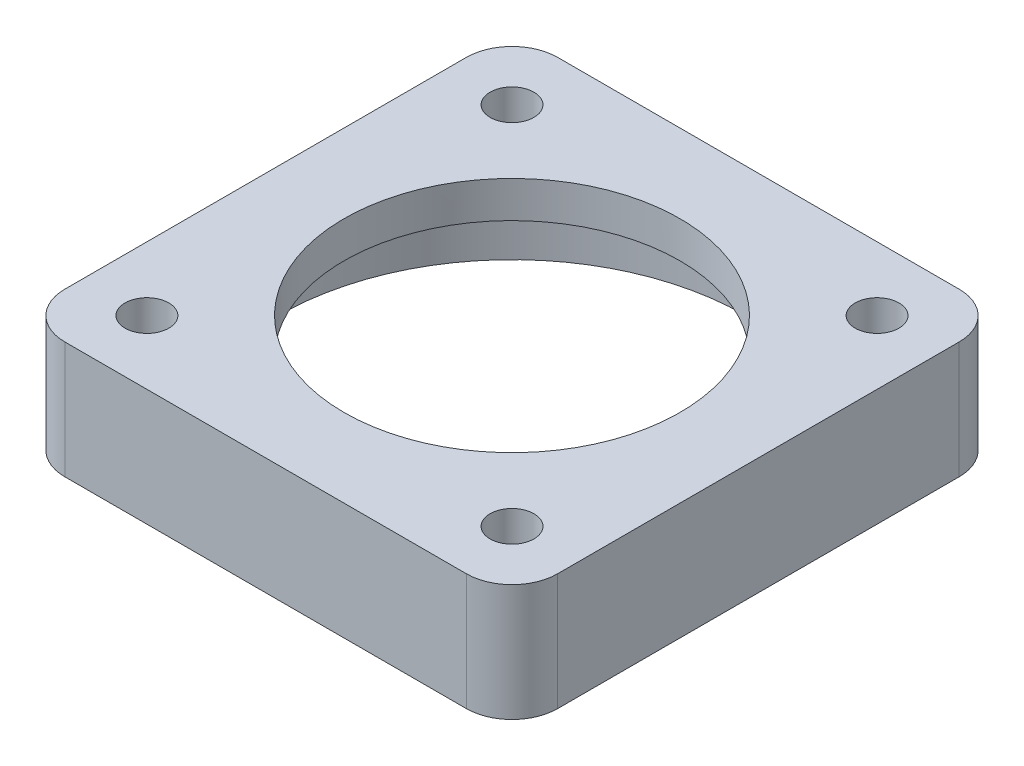
ISO-10303-21;
HEADER;
FILE_DESCRIPTION(('STEP AP214'),'2;1');
FILE_NAME('part.step','',(''),(''),'','','');
FILE_SCHEMA(('AUTOMOTIVE_DESIGN { 1 0 10303 214 1 1 1 1 }'));
ENDSEC;
DATA;
#1=APPLICATION_CONTEXT('core data for automotive mechanical design processes');
#2=APPLICATION_PROTOCOL_DEFINITION('international standard','automotive_design',2000,#1);
#3=PRODUCT_CONTEXT('',#1,'mechanical');
#4=PRODUCT('Part','Part','',(#3));
#5=PRODUCT_RELATED_PRODUCT_CATEGORY('part','',(#4));
#6=PRODUCT_DEFINITION_FORMATION('','',#4);
#7=PRODUCT_DEFINITION_CONTEXT('part definition',#1,'design');
#8=PRODUCT_DEFINITION('design','',#6,#7);
#9=PRODUCT_DEFINITION_SHAPE('','',#8);
#10=(LENGTH_UNIT() NAMED_UNIT(*) SI_UNIT(.MILLI.,.METRE.));
#11=(NAMED_UNIT(*) PLANE_ANGLE_UNIT() SI_UNIT($,.RADIAN.));
#12=(NAMED_UNIT(*) SI_UNIT($,.STERADIAN.) SOLID_ANGLE_UNIT());
#13=UNCERTAINTY_MEASURE_WITH_UNIT(LENGTH_MEASURE(1.E-05),#10,'distance_accuracy_value','');
#14=(GEOMETRIC_REPRESENTATION_CONTEXT(3) GLOBAL_UNCERTAINTY_ASSIGNED_CONTEXT((#13)) GLOBAL_UNIT_ASSIGNED_CONTEXT((#10,
#11,#12)) REPRESENTATION_CONTEXT('',''));
#15=CARTESIAN_POINT('',(0.,0.,0.));
#16=DIRECTION('',(0.,0.,1.));
#17=DIRECTION('',(1.,0.,0.));
#18=AXIS2_PLACEMENT_3D('',#15,#16,#17);
#19=CARTESIAN_POINT('',(0.,-0.001000000000001,0.));
#20=DIRECTION('',(0.,1.,0.));
#21=DIRECTION('',(0.,0.,1.));
#22=AXIS2_PLACEMENT_3D('',#19,#20,#21);
#23=CYLINDRICAL_SURFACE('',#22,46.);
#24=CARTESIAN_POINT('',(0.,32.,0.));
#25=DIRECTION('',(0.,1.,0.));
#26=DIRECTION('',(0.,0.,1.));
#27=AXIS2_PLACEMENT_3D('',#24,#25,#26);
#28=CIRCLE('',#27,46.);
#29=CARTESIAN_POINT('',(0.,32.,46.));
#30=VERTEX_POINT('',#29);
#31=EDGE_CURVE('E207',#30,#30,#28,.T.);
#32=ORIENTED_EDGE('',*,*,#31,.T.);
#33=EDGE_LOOP('',(#32));
#34=FACE_BOUND('',#33,.T.);
#35=CARTESIAN_POINT('',(0.,22.,0.));
#36=DIRECTION('',(0.,-1.,0.));
#37=DIRECTION('',(0.,0.,-1.));
#38=AXIS2_PLACEMENT_3D('',#35,#36,#37);
#39=CIRCLE('',#38,46.);
#40=CARTESIAN_POINT('',(0.,22.,-46.));
#41=VERTEX_POINT('',#40);
#42=EDGE_CURVE('E43',#41,#41,#39,.F.);
#43=ORIENTED_EDGE('',*,*,#42,.F.);
#44=EDGE_LOOP('',(#43));
#45=FACE_BOUND('',#44,.T.);
#46=ADVANCED_FACE('F39',(#34,#45),#23,.F.);
#47=CARTESIAN_POINT('',(-55.,32.,55.));
#48=DIRECTION('',(0.,1.,0.));
#49=DIRECTION('',(0.,0.,1.));
#50=AXIS2_PLACEMENT_3D('',#47,#48,#49);
#51=PLANE('',#50);
#52=ORIENTED_EDGE('',*,*,#31,.F.);
#53=EDGE_LOOP('',(#52));
#54=FACE_BOUND('',#53,.T.);
#55=CARTESIAN_POINT('',(50.0000000000001,32.,50.));
#56=DIRECTION('',(0.,1.,0.));
#57=DIRECTION('',(0.,0.,1.));
#58=AXIS2_PLACEMENT_3D('',#55,#56,#57);
#59=CIRCLE('',#58,5.99999999999999);
#60=CARTESIAN_POINT('',(50.0000000000001,32.,56.));
#61=VERTEX_POINT('',#60);
#62=EDGE_CURVE('E197',#61,#61,#59,.T.);
#63=ORIENTED_EDGE('',*,*,#62,.F.);
#64=EDGE_LOOP('',(#63));
#65=FACE_BOUND('',#64,.T.);
#66=CARTESIAN_POINT('',(-50.,32.,-50.));
#67=DIRECTION('',(0.,1.,0.));
#68=DIRECTION('',(0.,0.,1.));
#69=AXIS2_PLACEMENT_3D('',#66,#67,#68);
#70=CIRCLE('',#69,5.99999999999999);
#71=CARTESIAN_POINT('',(-50.,32.,-44.));
#72=VERTEX_POINT('',#71);
#73=EDGE_CURVE('E142',#72,#72,#70,.T.);
#74=ORIENTED_EDGE('',*,*,#73,.F.);
#75=EDGE_LOOP('',(#74));
#76=FACE_BOUND('',#75,.T.);
#77=CARTESIAN_POINT('',(-55.,32.,55.));
#78=DIRECTION('',(0.,1.,0.));
#79=DIRECTION('',(0.,0.,1.));
#80=AXIS2_PLACEMENT_3D('',#77,#78,#79);
#81=CIRCLE('',#80,12.5);
#82=CARTESIAN_POINT('',(-67.5,32.,55.));
#83=VERTEX_POINT('',#82);
#84=CARTESIAN_POINT('',(-55.,32.,67.5));
#85=VERTEX_POINT('',#84);
#86=EDGE_CURVE('E153',#83,#85,#81,.T.);
#87=ORIENTED_EDGE('',*,*,#86,.T.);
#88=DIRECTION('',(1.,0.,0.));
#89=VECTOR('',#88,1.);
#90=CARTESIAN_POINT('',(-55.,32.,67.5));
#91=LINE('',#90,#89);
#92=CARTESIAN_POINT('',(55.,32.,67.5));
#93=VERTEX_POINT('',#92);
#94=EDGE_CURVE('E99',#85,#93,#91,.T.);
#95=ORIENTED_EDGE('',*,*,#94,.T.);
#96=CARTESIAN_POINT('',(55.,32.,55.));
#97=DIRECTION('',(0.,1.,0.));
#98=DIRECTION('',(0.,0.,1.));
#99=AXIS2_PLACEMENT_3D('',#96,#97,#98);
#100=CIRCLE('',#99,12.5);
#101=CARTESIAN_POINT('',(67.5,32.,55.));
#102=VERTEX_POINT('',#101);
#103=EDGE_CURVE('E166',#93,#102,#100,.T.);
#104=ORIENTED_EDGE('',*,*,#103,.T.);
#105=DIRECTION('',(0.,0.,-1.));
#106=VECTOR('',#105,1.);
#107=CARTESIAN_POINT('',(67.5,32.,-55.));
#108=LINE('',#107,#106);
#109=CARTESIAN_POINT('',(67.5,32.,-55.));
#110=VERTEX_POINT('',#109);
#111=EDGE_CURVE('E185',#102,#110,#108,.T.);
#112=ORIENTED_EDGE('',*,*,#111,.T.);
#113=CARTESIAN_POINT('',(55.,32.,-55.));
#114=DIRECTION('',(0.,1.,0.));
#115=DIRECTION('',(0.,0.,1.));
#116=AXIS2_PLACEMENT_3D('',#113,#114,#115);
#117=CIRCLE('',#116,12.5);
#118=CARTESIAN_POINT('',(55.,32.,-67.5));
#119=VERTEX_POINT('',#118);
#120=EDGE_CURVE('E120',#110,#119,#117,.T.);
#121=ORIENTED_EDGE('',*,*,#120,.T.);
#122=DIRECTION('',(-1.,0.,0.));
#123=VECTOR('',#122,1.);
#124=CARTESIAN_POINT('',(-55.,32.,-67.5));
#125=LINE('',#124,#123);
#126=CARTESIAN_POINT('',(-55.,32.,-67.5));
#127=VERTEX_POINT('',#126);
#128=EDGE_CURVE('E114',#119,#127,#125,.T.);
#129=ORIENTED_EDGE('',*,*,#128,.T.);
#130=CARTESIAN_POINT('',(-55.,32.,-55.));
#131=DIRECTION('',(0.,1.,0.));
#132=DIRECTION('',(0.,0.,-1.));
#133=AXIS2_PLACEMENT_3D('',#130,#131,#132);
#134=CIRCLE('',#133,12.5);
#135=CARTESIAN_POINT('',(-67.5,32.,-55.));
#136=VERTEX_POINT('',#135);
#137=EDGE_CURVE('E119',#127,#136,#134,.T.);
#138=ORIENTED_EDGE('',*,*,#137,.T.);
#139=DIRECTION('',(0.,0.,1.));
#140=VECTOR('',#139,1.);
#141=CARTESIAN_POINT('',(-67.5,32.,-55.));
#142=LINE('',#141,#140);
#143=EDGE_CURVE('E60',#136,#83,#142,.T.);
#144=ORIENTED_EDGE('',*,*,#143,.T.);
#145=EDGE_LOOP('',(#87,#95,#104,#112,#121,#129,#138,#144));
#146=FACE_BOUND('',#145,.T.);
#147=CARTESIAN_POINT('',(50.,32.,-50.));
#148=DIRECTION('',(0.,1.,0.));
#149=DIRECTION('',(0.,0.,-1.));
#150=AXIS2_PLACEMENT_3D('',#147,#148,#149);
#151=CIRCLE('',#150,5.99999999999999);
#152=CARTESIAN_POINT('',(50.,32.,-56.));
#153=VERTEX_POINT('',#152);
#154=EDGE_CURVE('E191',#153,#153,#151,.T.);
#155=ORIENTED_EDGE('',*,*,#154,.F.);
#156=EDGE_LOOP('',(#155));
#157=FACE_BOUND('',#156,.T.);
#158=CARTESIAN_POINT('',(-49.9999999999998,32.,50.));
#159=DIRECTION('',(0.,1.,0.));
#160=DIRECTION('',(0.,0.,-1.));
#161=AXIS2_PLACEMENT_3D('',#158,#159,#160);
#162=CIRCLE('',#161,5.99999999999999);
#163=CARTESIAN_POINT('',(-49.9999999999998,32.,44.));
#164=VERTEX_POINT('',#163);
#165=EDGE_CURVE('E201',#164,#164,#162,.T.);
#166=ORIENTED_EDGE('',*,*,#165,.F.);
#167=EDGE_LOOP('',(#166));
#168=FACE_BOUND('',#167,.T.);
#169=ADVANCED_FACE('F113',(#54,#65,#76,#146,#157,#168),#51,.T.);
#170=CARTESIAN_POINT('',(-55.,0.,55.));
#171=DIRECTION('',(0.,1.,0.));
#172=DIRECTION('',(0.,0.,1.));
#173=AXIS2_PLACEMENT_3D('',#170,#171,#172);
#174=PLANE('',#173);
#175=CARTESIAN_POINT('',(0.,0.,0.));
#176=DIRECTION('',(0.,-1.,0.));
#177=DIRECTION('',(0.,0.,-1.));
#178=AXIS2_PLACEMENT_3D('',#175,#176,#177);
#179=CIRCLE('',#178,64.);
#180=CARTESIAN_POINT('',(0.,0.,-64.));
#181=VERTEX_POINT('',#180);
#182=EDGE_CURVE('E212',#181,#181,#179,.T.);
#183=ORIENTED_EDGE('',*,*,#182,.F.);
#184=EDGE_LOOP('',(#183));
#185=FACE_BOUND('',#184,.T.);
#186=CARTESIAN_POINT('',(-55.,0.,55.));
#187=DIRECTION('',(0.,1.,0.));
#188=DIRECTION('',(0.,0.,1.));
#189=AXIS2_PLACEMENT_3D('',#186,#187,#188);
#190=CIRCLE('',#189,12.5);
#191=CARTESIAN_POINT('',(-67.5,0.,55.));
#192=VERTEX_POINT('',#191);
#193=CARTESIAN_POINT('',(-55.,0.,67.5));
#194=VERTEX_POINT('',#193);
#195=EDGE_CURVE('E137',#192,#194,#190,.T.);
#196=ORIENTED_EDGE('',*,*,#195,.F.);
#197=DIRECTION('',(0.,0.,1.));
#198=VECTOR('',#197,1.);
#199=CARTESIAN_POINT('',(-67.5,0.,-55.));
#200=LINE('',#199,#198);
#201=CARTESIAN_POINT('',(-67.5,0.,-55.));
#202=VERTEX_POINT('',#201);
#203=EDGE_CURVE('E95',#202,#192,#200,.T.);
#204=ORIENTED_EDGE('',*,*,#203,.F.);
#205=CARTESIAN_POINT('',(-55.,0.,-55.));
#206=DIRECTION('',(0.,1.,0.));
#207=DIRECTION('',(0.,0.,-1.));
#208=AXIS2_PLACEMENT_3D('',#205,#206,#207);
#209=CIRCLE('',#208,12.5);
#210=CARTESIAN_POINT('',(-55.,0.,-67.5));
#211=VERTEX_POINT('',#210);
#212=EDGE_CURVE('E88',#211,#202,#209,.T.);
#213=ORIENTED_EDGE('',*,*,#212,.F.);
#214=DIRECTION('',(-1.,0.,0.));
#215=VECTOR('',#214,1.);
#216=CARTESIAN_POINT('',(-55.,0.,-67.5));
#217=LINE('',#216,#215);
#218=CARTESIAN_POINT('',(55.,0.,-67.5));
#219=VERTEX_POINT('',#218);
#220=EDGE_CURVE('E126',#219,#211,#217,.T.);
#221=ORIENTED_EDGE('',*,*,#220,.F.);
#222=CARTESIAN_POINT('',(55.,0.,-55.));
#223=DIRECTION('',(0.,1.,0.));
#224=DIRECTION('',(0.,0.,1.));
#225=AXIS2_PLACEMENT_3D('',#222,#223,#224);
#226=CIRCLE('',#225,12.5);
#227=CARTESIAN_POINT('',(67.5,0.,-55.));
#228=VERTEX_POINT('',#227);
#229=EDGE_CURVE('E146',#228,#219,#226,.T.);
#230=ORIENTED_EDGE('',*,*,#229,.F.);
#231=DIRECTION('',(0.,0.,-1.));
#232=VECTOR('',#231,1.);
#233=CARTESIAN_POINT('',(67.5,0.,-55.));
#234=LINE('',#233,#232);
#235=CARTESIAN_POINT('',(67.5,0.,55.));
#236=VERTEX_POINT('',#235);
#237=EDGE_CURVE('E148',#236,#228,#234,.T.);
#238=ORIENTED_EDGE('',*,*,#237,.F.);
#239=CARTESIAN_POINT('',(55.,0.,55.));
#240=DIRECTION('',(0.,1.,0.));
#241=DIRECTION('',(0.,0.,1.));
#242=AXIS2_PLACEMENT_3D('',#239,#240,#241);
#243=CIRCLE('',#242,12.5);
#244=CARTESIAN_POINT('',(55.,0.,67.5));
#245=VERTEX_POINT('',#244);
#246=EDGE_CURVE('E145',#245,#236,#243,.T.);
#247=ORIENTED_EDGE('',*,*,#246,.F.);
#248=DIRECTION('',(1.,0.,0.));
#249=VECTOR('',#248,1.);
#250=CARTESIAN_POINT('',(-55.,0.,67.5));
#251=LINE('',#250,#249);
#252=EDGE_CURVE('E143',#194,#245,#251,.T.);
#253=ORIENTED_EDGE('',*,*,#252,.F.);
#254=EDGE_LOOP('',(#196,#204,#213,#221,#230,#238,#247,#253));
#255=FACE_BOUND('',#254,.T.);
#256=CARTESIAN_POINT('',(-50.,0.,-50.));
#257=DIRECTION('',(0.,1.,0.));
#258=DIRECTION('',(0.,0.,1.));
#259=AXIS2_PLACEMENT_3D('',#256,#257,#258);
#260=CIRCLE('',#259,5.99999999999999);
#261=CARTESIAN_POINT('',(-50.,0.,-44.));
#262=VERTEX_POINT('',#261);
#263=EDGE_CURVE('E189',#262,#262,#260,.T.);
#264=ORIENTED_EDGE('',*,*,#263,.T.);
#265=EDGE_LOOP('',(#264));
#266=FACE_BOUND('',#265,.T.);
#267=CARTESIAN_POINT('',(50.,0.,-50.));
#268=DIRECTION('',(0.,1.,0.));
#269=DIRECTION('',(0.,0.,-1.));
#270=AXIS2_PLACEMENT_3D('',#267,#268,#269);
#271=CIRCLE('',#270,5.99999999999999);
#272=CARTESIAN_POINT('',(50.,0.,-56.));
#273=VERTEX_POINT('',#272);
#274=EDGE_CURVE('E193',#273,#273,#271,.T.);
#275=ORIENTED_EDGE('',*,*,#274,.T.);
#276=EDGE_LOOP('',(#275));
#277=FACE_BOUND('',#276,.T.);
#278=CARTESIAN_POINT('',(50.0000000000001,0.,50.));
#279=DIRECTION('',(0.,1.,0.));
#280=DIRECTION('',(0.,0.,1.));
#281=AXIS2_PLACEMENT_3D('',#278,#279,#280);
#282=CIRCLE('',#281,5.99999999999999);
#283=CARTESIAN_POINT('',(50.0000000000001,0.,56.));
#284=VERTEX_POINT('',#283);
#285=EDGE_CURVE('E199',#284,#284,#282,.T.);
#286=ORIENTED_EDGE('',*,*,#285,.T.);
#287=EDGE_LOOP('',(#286));
#288=FACE_BOUND('',#287,.T.);
#289=CARTESIAN_POINT('',(-49.9999999999998,0.,50.));
#290=DIRECTION('',(0.,1.,0.));
#291=DIRECTION('',(0.,0.,-1.));
#292=AXIS2_PLACEMENT_3D('',#289,#290,#291);
#293=CIRCLE('',#292,5.99999999999999);
#294=CARTESIAN_POINT('',(-49.9999999999998,0.,44.));
#295=VERTEX_POINT('',#294);
#296=EDGE_CURVE('E206',#295,#295,#293,.T.);
#297=ORIENTED_EDGE('',*,*,#296,.T.);
#298=EDGE_LOOP('',(#297));
#299=FACE_BOUND('',#298,.T.);
#300=ADVANCED_FACE('F174',(#185,#255,#266,#277,#288,#299),#174,.F.);
#301=CARTESIAN_POINT('',(-55.,32.,55.));
#302=DIRECTION('',(0.,-1.,0.));
#303=DIRECTION('',(0.,0.,-1.));
#304=AXIS2_PLACEMENT_3D('',#301,#302,#303);
#305=CYLINDRICAL_SURFACE('',#304,12.5);
#306=ORIENTED_EDGE('',*,*,#195,.T.);
#307=DIRECTION('',(0.,-1.,0.));
#308=VECTOR('',#307,1.);
#309=CARTESIAN_POINT('',(-55.,32.,67.5));
#310=LINE('',#309,#308);
#311=EDGE_CURVE('E11',#85,#194,#310,.T.);
#312=ORIENTED_EDGE('',*,*,#311,.F.);
#313=ORIENTED_EDGE('',*,*,#86,.F.);
#314=DIRECTION('',(0.,-1.,0.));
#315=VECTOR('',#314,1.);
#316=CARTESIAN_POINT('',(-67.5,32.,55.));
#317=LINE('',#316,#315);
#318=EDGE_CURVE('E133',#83,#192,#317,.T.);
#319=ORIENTED_EDGE('',*,*,#318,.T.);
#320=EDGE_LOOP('',(#306,#312,#313,#319));
#321=FACE_BOUND('',#320,.T.);
#322=ADVANCED_FACE('F41',(#321),#305,.T.);
#323=CARTESIAN_POINT('',(-55.,32.,67.5));
#324=DIRECTION('',(0.,0.,-1.));
#325=DIRECTION('',(-1.,0.,0.));
#326=AXIS2_PLACEMENT_3D('',#323,#324,#325);
#327=PLANE('',#326);
#328=ORIENTED_EDGE('',*,*,#252,.T.);
#329=DIRECTION('',(0.,-1.,0.));
#330=VECTOR('',#329,1.);
#331=CARTESIAN_POINT('',(55.,32.,67.5));
#332=LINE('',#331,#330);
#333=EDGE_CURVE('E47',#93,#245,#332,.T.);
#334=ORIENTED_EDGE('',*,*,#333,.F.);
#335=ORIENTED_EDGE('',*,*,#94,.F.);
#336=ORIENTED_EDGE('',*,*,#311,.T.);
#337=EDGE_LOOP('',(#328,#334,#335,#336));
#338=FACE_BOUND('',#337,.T.);
#339=ADVANCED_FACE('F267',(#338),#327,.F.);
#340=CARTESIAN_POINT('',(55.,32.,55.));
#341=DIRECTION('',(0.,-1.,0.));
#342=DIRECTION('',(0.,0.,-1.));
#343=AXIS2_PLACEMENT_3D('',#340,#341,#342);
#344=CYLINDRICAL_SURFACE('',#343,12.5);
#345=ORIENTED_EDGE('',*,*,#246,.T.);
#346=DIRECTION('',(0.,-1.,0.));
#347=VECTOR('',#346,1.);
#348=CARTESIAN_POINT('',(67.5,32.,55.));
#349=LINE('',#348,#347);
#350=EDGE_CURVE('E159',#102,#236,#349,.T.);
#351=ORIENTED_EDGE('',*,*,#350,.F.);
#352=ORIENTED_EDGE('',*,*,#103,.F.);
#353=ORIENTED_EDGE('',*,*,#333,.T.);
#354=EDGE_LOOP('',(#345,#351,#352,#353));
#355=FACE_BOUND('',#354,.T.);
#356=ADVANCED_FACE('F170',(#355),#344,.T.);
#357=CARTESIAN_POINT('',(67.5,32.,-55.));
#358=DIRECTION('',(-1.,0.,0.));
#359=DIRECTION('',(0.,0.,1.));
#360=AXIS2_PLACEMENT_3D('',#357,#358,#359);
#361=PLANE('',#360);
#362=ORIENTED_EDGE('',*,*,#237,.T.);
#363=DIRECTION('',(0.,-1.,0.));
#364=VECTOR('',#363,1.);
#365=CARTESIAN_POINT('',(67.5,32.,-55.));
#366=LINE('',#365,#364);
#367=EDGE_CURVE('E160',#110,#228,#366,.T.);
#368=ORIENTED_EDGE('',*,*,#367,.F.);
#369=ORIENTED_EDGE('',*,*,#111,.F.);
#370=ORIENTED_EDGE('',*,*,#350,.T.);
#371=EDGE_LOOP('',(#362,#368,#369,#370));
#372=FACE_BOUND('',#371,.T.);
#373=ADVANCED_FACE('F177',(#372),#361,.F.);
#374=CARTESIAN_POINT('',(55.,32.,-55.));
#375=DIRECTION('',(0.,-1.,0.));
#376=DIRECTION('',(0.,0.,-1.));
#377=AXIS2_PLACEMENT_3D('',#374,#375,#376);
#378=CYLINDRICAL_SURFACE('',#377,12.5);
#379=ORIENTED_EDGE('',*,*,#229,.T.);
#380=DIRECTION('',(0.,-1.,0.));
#381=VECTOR('',#380,1.);
#382=CARTESIAN_POINT('',(55.,32.,-67.5));
#383=LINE('',#382,#381);
#384=EDGE_CURVE('E129',#119,#219,#383,.T.);
#385=ORIENTED_EDGE('',*,*,#384,.F.);
#386=ORIENTED_EDGE('',*,*,#120,.F.);
#387=ORIENTED_EDGE('',*,*,#367,.T.);
#388=EDGE_LOOP('',(#379,#385,#386,#387));
#389=FACE_BOUND('',#388,.T.);
#390=ADVANCED_FACE('F182',(#389),#378,.T.);
#391=CARTESIAN_POINT('',(-55.,32.,-67.5));
#392=DIRECTION('',(0.,0.,1.));
#393=DIRECTION('',(1.,0.,0.));
#394=AXIS2_PLACEMENT_3D('',#391,#392,#393);
#395=PLANE('',#394);
#396=ORIENTED_EDGE('',*,*,#220,.T.);
#397=DIRECTION('',(0.,-1.,0.));
#398=VECTOR('',#397,1.);
#399=CARTESIAN_POINT('',(-55.,32.,-67.5));
#400=LINE('',#399,#398);
#401=EDGE_CURVE('E124',#127,#211,#400,.T.);
#402=ORIENTED_EDGE('',*,*,#401,.F.);
#403=ORIENTED_EDGE('',*,*,#128,.F.);
#404=ORIENTED_EDGE('',*,*,#384,.T.);
#405=EDGE_LOOP('',(#396,#402,#403,#404));
#406=FACE_BOUND('',#405,.T.);
#407=ADVANCED_FACE('F127',(#406),#395,.F.);
#408=CARTESIAN_POINT('',(-55.,32.,-55.));
#409=DIRECTION('',(0.,-1.,0.));
#410=DIRECTION('',(0.,0.,-1.));
#411=AXIS2_PLACEMENT_3D('',#408,#409,#410);
#412=CYLINDRICAL_SURFACE('',#411,12.5);
#413=ORIENTED_EDGE('',*,*,#212,.T.);
#414=DIRECTION('',(0.,-1.,0.));
#415=VECTOR('',#414,1.);
#416=CARTESIAN_POINT('',(-67.5,32.,-55.));
#417=LINE('',#416,#415);
#418=EDGE_CURVE('E128',#136,#202,#417,.T.);
#419=ORIENTED_EDGE('',*,*,#418,.F.);
#420=ORIENTED_EDGE('',*,*,#137,.F.);
#421=ORIENTED_EDGE('',*,*,#401,.T.);
#422=EDGE_LOOP('',(#413,#419,#420,#421));
#423=FACE_BOUND('',#422,.T.);
#424=ADVANCED_FACE('F132',(#423),#412,.T.);
#425=CARTESIAN_POINT('',(-67.5,32.,-55.));
#426=DIRECTION('',(1.,0.,0.));
#427=DIRECTION('',(0.,0.,-1.));
#428=AXIS2_PLACEMENT_3D('',#425,#426,#427);
#429=PLANE('',#428);
#430=ORIENTED_EDGE('',*,*,#203,.T.);
#431=ORIENTED_EDGE('',*,*,#318,.F.);
#432=ORIENTED_EDGE('',*,*,#143,.F.);
#433=ORIENTED_EDGE('',*,*,#418,.T.);
#434=EDGE_LOOP('',(#430,#431,#432,#433));
#435=FACE_BOUND('',#434,.T.);
#436=ADVANCED_FACE('F251',(#435),#429,.F.);
#437=CARTESIAN_POINT('',(-50.,32.,-50.));
#438=DIRECTION('',(0.,-1.,0.));
#439=DIRECTION('',(0.,0.,-1.));
#440=AXIS2_PLACEMENT_3D('',#437,#438,#439);
#441=CYLINDRICAL_SURFACE('',#440,5.99999999999999);
#442=ORIENTED_EDGE('',*,*,#73,.T.);
#443=EDGE_LOOP('',(#442));
#444=FACE_BOUND('',#443,.T.);
#445=ORIENTED_EDGE('',*,*,#263,.F.);
#446=EDGE_LOOP('',(#445));
#447=FACE_BOUND('',#446,.T.);
#448=ADVANCED_FACE('F249',(#444,#447),#441,.F.);
#449=CARTESIAN_POINT('',(50.,32.,-50.));
#450=DIRECTION('',(0.,-1.,0.));
#451=DIRECTION('',(0.,0.,-1.));
#452=AXIS2_PLACEMENT_3D('',#449,#450,#451);
#453=CYLINDRICAL_SURFACE('',#452,5.99999999999999);
#454=ORIENTED_EDGE('',*,*,#154,.T.);
#455=EDGE_LOOP('',(#454));
#456=FACE_BOUND('',#455,.T.);
#457=ORIENTED_EDGE('',*,*,#274,.F.);
#458=EDGE_LOOP('',(#457));
#459=FACE_BOUND('',#458,.T.);
#460=ADVANCED_FACE('F246',(#456,#459),#453,.F.);
#461=CARTESIAN_POINT('',(50.0000000000001,32.,50.));
#462=DIRECTION('',(0.,-1.,0.));
#463=DIRECTION('',(0.,0.,-1.));
#464=AXIS2_PLACEMENT_3D('',#461,#462,#463);
#465=CYLINDRICAL_SURFACE('',#464,5.99999999999999);
#466=ORIENTED_EDGE('',*,*,#62,.T.);
#467=EDGE_LOOP('',(#466));
#468=FACE_BOUND('',#467,.T.);
#469=ORIENTED_EDGE('',*,*,#285,.F.);
#470=EDGE_LOOP('',(#469));
#471=FACE_BOUND('',#470,.T.);
#472=ADVANCED_FACE('F242',(#468,#471),#465,.F.);
#473=CARTESIAN_POINT('',(-49.9999999999998,32.,50.));
#474=DIRECTION('',(0.,-1.,0.));
#475=DIRECTION('',(0.,0.,-1.));
#476=AXIS2_PLACEMENT_3D('',#473,#474,#475);
#477=CYLINDRICAL_SURFACE('',#476,5.99999999999999);
#478=ORIENTED_EDGE('',*,*,#165,.T.);
#479=EDGE_LOOP('',(#478));
#480=FACE_BOUND('',#479,.T.);
#481=ORIENTED_EDGE('',*,*,#296,.F.);
#482=EDGE_LOOP('',(#481));
#483=FACE_BOUND('',#482,.T.);
#484=ADVANCED_FACE('F239',(#480,#483),#477,.F.);
#485=CARTESIAN_POINT('',(0.,22.,0.));
#486=DIRECTION('',(0.,-1.,0.));
#487=DIRECTION('',(0.,0.,-1.));
#488=AXIS2_PLACEMENT_3D('',#485,#486,#487);
#489=PLANE('',#488);
#490=CARTESIAN_POINT('',(0.,22.,0.));
#491=DIRECTION('',(0.,-1.,0.));
#492=DIRECTION('',(0.,0.,-1.));
#493=AXIS2_PLACEMENT_3D('',#490,#491,#492);
#494=CIRCLE('',#493,64.);
#495=CARTESIAN_POINT('',(0.,22.,-64.));
#496=VERTEX_POINT('',#495);
#497=EDGE_CURVE('E220',#496,#496,#494,.T.);
#498=ORIENTED_EDGE('',*,*,#497,.T.);
#499=EDGE_LOOP('',(#498));
#500=FACE_BOUND('',#499,.T.);
#501=ORIENTED_EDGE('',*,*,#42,.T.);
#502=EDGE_LOOP('',(#501));
#503=FACE_BOUND('',#502,.T.);
#504=ADVANCED_FACE('F221',(#500,#503),#489,.T.);
#505=CARTESIAN_POINT('',(0.,22.,0.));
#506=DIRECTION('',(0.,-1.,0.));
#507=DIRECTION('',(0.,0.,-1.));
#508=AXIS2_PLACEMENT_3D('',#505,#506,#507);
#509=CYLINDRICAL_SURFACE('',#508,64.);
#510=ORIENTED_EDGE('',*,*,#497,.F.);
#511=EDGE_LOOP('',(#510));
#512=FACE_BOUND('',#511,.T.);
#513=ORIENTED_EDGE('',*,*,#182,.T.);
#514=EDGE_LOOP('',(#513));
#515=FACE_BOUND('',#514,.T.);
#516=ADVANCED_FACE('F240',(#512,#515),#509,.F.);
#517=CLOSED_SHELL('',(#46,#169,#300,#322,#339,#356,#373,#390,#407,#424,#436,#448,#460,#472,#484,
#504,#516));
#518=MANIFOLD_SOLID_BREP('B2',#517);
#519=ADVANCED_BREP_SHAPE_REPRESENTATION('',(#18,#518),#14);
#520=SHAPE_DEFINITION_REPRESENTATION(#9,#519);
ENDSEC;
END-ISO-10303-21;
